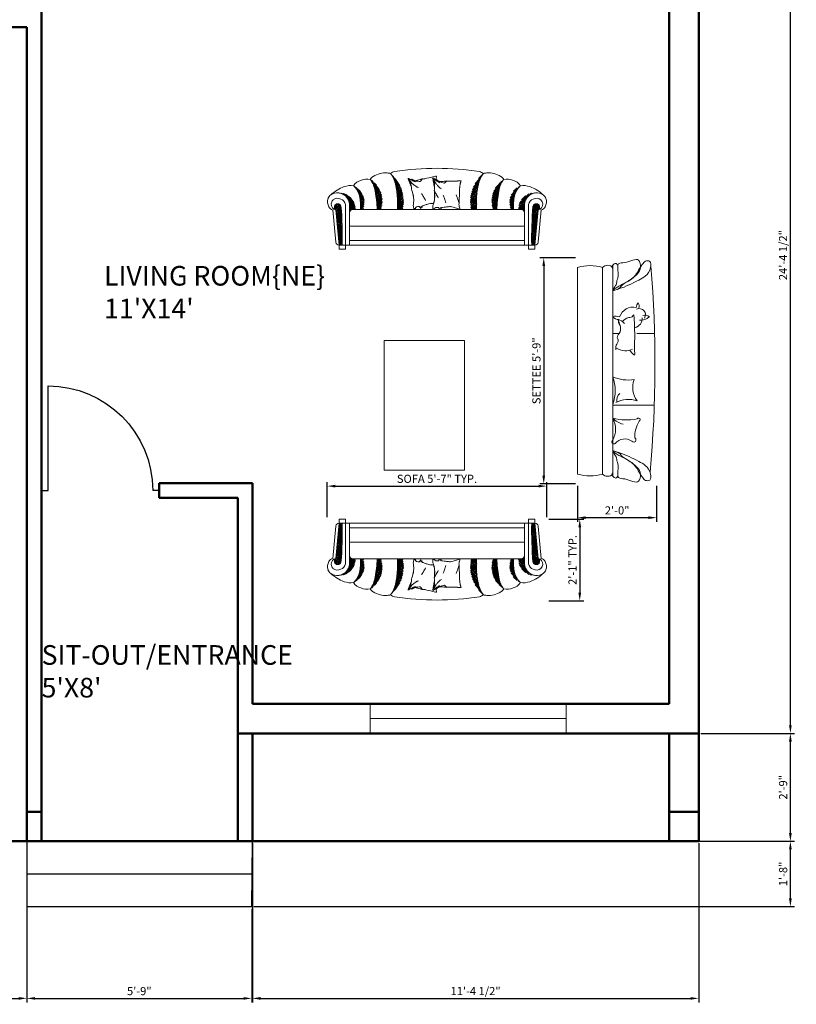
# Model space of a CAD drawing. Units: inches. Extents: x 20697 to 21575, y 6189 to 6822.
# Tile 2 of 7: x 20826 to 21063, y 6189 to 6490. Entities that reach past the tile are written whole.
import ezdxf

# ---------------------------------------------------------------- set-up
doc = ezdxf.new("R2010")
doc.units = ezdxf.units.IN
for name, color, linetype, lineweight in [('A-ANNO-DIMS', 2, 'Continuous', 18), ('A-AREA-IDEN', 7, 'Continuous', 18), ('A-DOOR', 4, 'Continuous', 25), ('A-FLOR-STRS', 3, 'Continuous', 25), ('A-FURN', 8, 'Continuous', 18), ('A-GLAZ', 4, 'Continuous', 18), ('A-WALL', 7, 'Continuous', 50)]:
    doc.layers.add(name, color=color, linetype=linetype, lineweight=lineweight)
doc.styles.get("Standard").update_dxf_attribs({"font": 'arial.ttf'})
doc.dimstyles.new('ISO-25', dxfattribs={"dimtxt": 2.5, "dimasz": 2.5, "dimexe": 1.25, "dimexo": 0.625, "dimtad": 1, "dimdec": 0, "dimlunit": 3, "dimtxsty": 'Standard', "dimcen": 2.5, "dimadec": 0, "dimazin": 0, "dimtfac": 1, "dimtdec": 0, "dimtmove": 0, "dimatfit": 3, "dimfxl": 1, "dimarcsym": 0})

# ---------------------------------------------------------------- blocks, each defined once
blk = doc.blocks.new('A$C37157CB5')
for p, q in [((460, 748), (461, 749)), ((467, 737), (471, 741)), ((489, 723), (470, 742)), ((680, 808), (681, 809)), ((687, 798), (690, 801)), ((694, 787), (699, 792)), ((710, 768), (699, 778)), ((701, 776), (708, 783)), ((706, 764), (716, 774)), ((712, 752), (724, 764)), ((719, 741), (715, 745)), ((717, 739), (732, 755)), ((721, 726), (740, 745)), ((745, 732), (723, 754)), ((1586, 707), (1643, 765)), ((1630, 731), (1615, 746)), ((1629, 750), (1620, 758)), ((1624, 763), (1670, 809)), ((1640, 757), (1633, 763)), ((1645, 769), (1636, 778)), ((1651, 780), (1651, 781)), ((1658, 791), (1654, 796)), ((1672, 812), (1672, 812)), ((1803, 660), (1885, 741)), ((1885, 741), (1882, 744)), ((284, 678), (286, 679)), ((294, 670), (286, 679)), ((292, 668), (297, 673)), ((300, 659), (308, 666)), ((308, 649), (318, 659)), ((330, 635), (308, 657)), ((315, 638), (328, 650)), ((322, 627), (337, 642)), ((474, 726), (481, 734)), ((481, 715), (491, 726)), ((498, 697), (482, 713)), ((487, 703), (500, 717)), ((492, 691), (509, 708)), ((507, 670), (496, 681)), ((497, 679), (518, 699)), ((524, 688), (502, 710)), ((502, 665), (526, 689)), ((515, 644), (505, 655)), ((506, 652), (533, 679)), ((509, 637), (540, 669)), ((533, 662), (511, 684)), ((512, 622), (547, 658)), ((514, 607), (553, 647)), ((516, 592), (559, 635)), ((542, 635), (520, 657)), ((559, 636), (546, 648)), ((728, 715), (724, 719)), ((725, 712), (747, 734)), ((728, 698), (754, 723)), ((736, 688), (729, 696)), ((731, 683), (761, 712)), ((754, 706), (732, 728)), ((745, 662), (733, 674)), ((734, 668), (767, 701)), ((737, 654), (773, 690)), ((754, 635), (738, 652)), ((740, 639), (779, 678)), ((763, 679), (741, 701)), ((742, 623), (784, 665)), ((744, 608), (789, 653)), ((746, 592), (794, 640)), ((772, 653), (750, 675)), ((781, 626), (759, 648)), ((776, 684), (767, 693)), ((789, 653), (776, 666)), ((798, 626), (785, 640)), ((1539, 572), (1610, 643)), ((1543, 593), (1614, 665)), ((1548, 617), (1619, 688)), ((1556, 642), (1624, 710)), ((1576, 626), (1557, 645)), ((1567, 653), (1562, 658)), ((1568, 671), (1631, 735)), ((1593, 644), (1571, 666)), ((1584, 670), (1573, 682)), ((1602, 617), (1580, 640)), ((1602, 688), (1585, 706)), ((1611, 662), (1589, 684)), ((1593, 715), (1591, 717)), ((1620, 706), (1598, 728)), ((1611, 644), (1598, 657)), ((1611, 732), (1605, 738)), ((1619, 689), (1607, 701)), ((1616, 674), (1615, 675)), ((1626, 718), (1624, 719)), ((1770, 573), (1843, 646)), ((1776, 596), (1850, 670)), ((1785, 624), (1861, 700)), ((1814, 617), (1792, 639)), ((1805, 644), (1798, 651)), ((1832, 635), (1810, 657)), ((1823, 662), (1812, 673)), ((1841, 679), (1827, 693)), ((1845, 657), (1828, 675)), ((1842, 643), (1836, 648)), ((1858, 697), (1844, 712)), ((1854, 683), (1845, 693)), ((1871, 719), (1862, 729)), ((1865, 708), (1863, 710)), ((1972, 580), (2046, 655)), ((1996, 622), (2034, 660)), ((2024, 620), (2008, 636)), ((2018, 644), (2016, 645)), ((2037, 642), (2026, 654)), ((2052, 662), (2046, 669)), ((2069, 681), (2068, 681)), ((122, 604), (123, 605)), ((136, 601), (140, 604)), ((153, 600), (150, 603)), ((150, 596), (156, 602)), ((162, 591), (170, 599)), ((180, 591), (172, 599)), ((174, 585), (184, 595)), ((184, 578), (196, 590)), ((215, 556), (193, 578)), ((194, 570), (208, 584)), ((206, 582), (200, 589)), ((203, 561), (219, 578)), ((211, 551), (230, 570)), ((218, 541), (240, 563)), ((241, 547), (219, 569)), ((224, 529), (222, 531)), ((223, 528), (249, 554)), ((228, 515), (257, 545)), ((250, 520), (228, 542)), ((232, 502), (265, 535)), ((277, 511), (255, 533)), ((339, 609), (323, 625)), ((327, 615), (345, 633)), ((333, 603), (353, 623)), ((348, 582), (336, 593)), ((338, 590), (360, 613)), ((342, 576), (367, 602)), ((365, 600), (343, 622)), ((356, 556), (343, 569)), ((345, 562), (373, 590)), ((347, 546), (379, 578)), ((365, 529), (347, 547)), ((349, 531), (384, 565)), ((351, 515), (388, 552)), ((374, 573), (352, 595)), ((353, 499), (391, 537)), ((383, 547), (361, 569)), ((392, 520), (370, 542)), ((524, 617), (510, 632)), ((533, 591), (513, 611)), ((519, 577), (565, 623)), ((542, 564), (520, 586)), ((521, 561), (570, 610)), ((523, 545), (574, 596)), ((524, 547), (523, 548)), ((525, 530), (578, 582)), ((527, 514), (581, 568)), ((528, 498), (583, 553)), ((551, 609), (529, 631)), ((551, 538), (529, 560)), ((530, 481), (585, 537)), ((560, 582), (538, 604)), ((560, 511), (538, 533)), ((568, 556), (546, 578)), ((571, 606), (555, 622)), ((577, 529), (555, 551)), ((578, 581), (564, 595)), ((582, 559), (573, 569)), ((585, 539), (582, 542)), ((763, 609), (741, 630)), ((748, 575), (798, 626)), ((754, 564), (748, 571)), ((749, 559), (802, 613)), ((749, 542), (806, 598)), ((749, 506), (811, 568)), ((749, 489), (813, 553)), ((763, 538), (749, 552)), ((749, 471), (815, 536)), ((772, 582), (750, 604)), ((750, 524), (809, 584)), ((772, 511), (750, 533)), ((781, 556), (759, 578)), ((789, 600), (767, 622)), ((789, 529), (767, 551)), ((798, 573), (776, 595)), ((807, 547), (785, 569)), ((805, 602), (794, 613)), ((815, 521), (794, 542)), ((809, 580), (803, 586)), ((813, 559), (812, 560)), ((1534, 514), (1603, 583)), ((1534, 497), (1601, 563)), ((1535, 532), (1605, 602)), ((1535, 480), (1600, 545)), ((1536, 551), (1607, 622)), ((1558, 538), (1537, 559)), ((1549, 564), (1539, 574)), ((1567, 582), (1545, 604)), ((1567, 511), (1545, 533)), ((1558, 609), (1549, 618)), ((1576, 556), (1554, 578)), ((1584, 600), (1562, 622)), ((1584, 529), (1562, 551)), ((1593, 573), (1571, 595)), ((1600, 548), (1580, 569)), ((1604, 598), (1589, 613)), ((1600, 531), (1589, 542)), ((1602, 582), (1598, 586)), ((1608, 629), (1607, 631)), ((1764, 532), (1835, 603)), ((1764, 514), (1832, 582)), ((1765, 497), (1829, 561)), ((1770, 538), (1765, 543)), ((1766, 552), (1838, 624)), ((1766, 481), (1826, 541)), ((1788, 556), (1770, 574)), ((1779, 582), (1773, 588)), ((1797, 529), (1774, 551)), ((1797, 600), (1782, 615)), ((1805, 573), (1783, 595)), ((1788, 626), (1787, 627)), ((1814, 547), (1792, 569)), ((1823, 591), (1801, 613)), ((1823, 520), (1801, 542)), ((1829, 567), (1810, 586)), ((1836, 613), (1819, 631)), ((1827, 551), (1819, 560)), ((1834, 598), (1828, 604)), ((1956, 512), (2005, 560)), ((1956, 494), (2001, 539)), ((1958, 531), (2010, 583)), ((1962, 553), (2020, 611)), ((1982, 538), (1963, 557)), ((1973, 564), (1968, 570)), ((1991, 511), (1969, 533)), ((1991, 582), (1978, 595)), ((2000, 556), (1978, 578)), ((2001, 537), (1987, 551)), ((2009, 600), (1992, 617)), ((2009, 581), (1995, 595)), ((2000, 626), (1999, 627)), ((2006, 567), (2004, 569)), ((2019, 607), (2013, 613)), ((2055, 469), (2148, 562)), ((2062, 494), (2162, 594)), ((2082, 532), (2124, 574)), ((2106, 520), (2087, 539)), ((2097, 547), (2095, 548)), ((2124, 538), (2104, 557)), ((2123, 520), (2110, 533)), ((2115, 564), (2114, 566)), ((2141, 556), (2124, 573)), ((2134, 545), (2128, 551)), ((2159, 573), (2146, 587)), ((2150, 564), (2146, 569)), ((2153, 567), (2187, 601)), ((2169, 581), (2163, 586)), ((2177, 591), (2171, 597)), ((2192, 593), (2185, 601)), ((2200, 597), (2208, 604)), ((2218, 602), (2216, 605)), ((2224, 603), (2226, 605)), ((75, 451), (110, 486)), ((91, 432), (75, 448)), ((82, 458), (77, 464)), ((78, 436), (124, 482)), ((85, 426), (134, 475)), ((109, 449), (87, 472)), ((91, 414), (142, 464)), ((92, 397), (144, 450)), ((100, 476), (94, 482)), ((94, 381), (145, 433)), ((118, 423), (96, 445)), ((127, 467), (108, 485)), ((135, 441), (113, 463)), ((144, 414), (122, 436)), ((144, 449), (140, 454)), ((191, 481), (191, 45)), ((233, 503), (231, 504)), ((234, 487), (272, 524)), ((241, 476), (235, 482)), ((236, 471), (279, 513)), ((236, 453), (284, 501)), ((236, 435), (289, 489)), ((236, 418), (293, 475)), ((250, 449), (236, 464)), ((236, 45), (236, 461)), ((259, 494), (237, 516)), ((257, 425), (237, 445)), ((268, 467), (246, 489)), ((277, 441), (255, 463)), ((263, 427), (296, 460)), ((286, 485), (264, 507)), ((272, 427), (264, 436)), ((270, 427), (2080, 427)), ((294, 458), (272, 480)), ((299, 437), (281, 454)), ((281, 427), (298, 444)), ((374, 503), (352, 525)), ((356, 485), (353, 488)), ((354, 482), (393, 521)), ((354, 465), (394, 505)), ((354, 448), (393, 486)), ((365, 458), (354, 469)), ((354, 430), (390, 466)), ((374, 432), (354, 451)), ((383, 476), (361, 498)), ((388, 454), (370, 472)), ((370, 427), (384, 442)), ((394, 500), (378, 516)), ((384, 440), (378, 445)), ((393, 484), (387, 489)), ((533, 520), (525, 528)), ((542, 494), (527, 509)), ((551, 467), (529, 489)), ((531, 465), (586, 520)), ((532, 448), (585, 502)), ((533, 449), (532, 451)), ((533, 432), (583, 482)), ((537, 427), (533, 432)), ((560, 441), (538, 463)), ((568, 485), (546, 507)), ((555, 427), (546, 436)), ((547, 427), (580, 461)), ((577, 458), (555, 480)), ((585, 503), (564, 525)), ((576, 442), (564, 454)), ((564, 427), (574, 437)), ((584, 487), (573, 498)), ((582, 471), (582, 472)), ((749, 454), (815, 519)), ((754, 494), (749, 499)), ((763, 467), (749, 481)), ((750, 436), (815, 502)), ((772, 441), (750, 463)), ((781, 485), (759, 507)), ((759, 427), (814, 483)), ((767, 427), (759, 436)), ((789, 458), (767, 480)), ((798, 503), (776, 525)), ((776, 427), (812, 464)), ((798, 432), (776, 454)), ((807, 476), (785, 498)), ((811, 454), (794, 472)), ((794, 427), (809, 443)), ((815, 503), (803, 516)), ((809, 439), (803, 445)), ((815, 486), (812, 489)), ((1003, 462, 12021), (1013, 456, 12021)), ((1137, 491), (1113, 493)), ((1211, 447, 12021), (1220, 439, 12021)), ((1394, 438), (1325, 458)), ((1419, 432), (1394, 438)), ((1540, 520), (1534, 526)), ((1549, 494), (1534, 509)), ((1558, 467), (1536, 489)), ((1537, 464), (1600, 527)), ((1539, 448), (1600, 510)), ((1540, 449), (1539, 451)), ((1542, 434), (1601, 492)), ((1545, 427), (1543, 429)), ((1567, 441), (1545, 463)), ((1576, 485), (1554, 507)), ((1554, 427), (1600, 474)), ((1562, 427), (1554, 436)), ((1584, 458), (1562, 480)), ((1593, 503), (1571, 525)), ((1571, 427), (1600, 456)), ((1593, 432), (1571, 454)), ((1601, 478), (1580, 498)), ((1600, 460), (1589, 472)), ((1589, 427), (1600, 438)), ((1600, 513), (1598, 516)), ((1600, 443), (1598, 445)), ((1779, 511), (1764, 526)), ((1788, 485), (1766, 507)), ((1770, 467), (1768, 469)), ((1769, 466), (1824, 521)), ((1772, 451), (1822, 501)), ((1779, 441), (1773, 447)), ((1797, 458), (1774, 480)), ((1776, 437), (1820, 482)), ((1805, 503), (1783, 525)), ((1783, 427), (1818, 462)), ((1805, 432), (1783, 454)), ((1814, 476), (1792, 498)), ((1818, 455), (1801, 472)), ((1801, 427), (1817, 443)), ((1822, 504), (1810, 516)), ((1817, 438), (1810, 445)), ((1820, 488), (1819, 489)), ((1973, 494), (1956, 511)), ((1965, 520), (1957, 527)), ((1957, 478), (1999, 519)), ((1960, 462), (1997, 500)), ((1982, 467), (1960, 489)), ((1965, 449), (1962, 452)), ((1963, 448), (1996, 481)), ((1968, 435), (1995, 462)), ((1991, 441), (1969, 463)), ((1996, 489), (1978, 507)), ((1978, 427), (1995, 445)), ((1986, 427), (1978, 436)), ((1995, 472), (1987, 480)), ((1999, 521), (1995, 525)), ((2051, 430), (2117, 495)), ((2057, 427), (2051, 434)), ((2052, 448), (2123, 520)), ((2062, 441), (2052, 451)), ((2079, 458), (2058, 480)), ((2071, 485), (2062, 494)), ((2066, 427), (2114, 475)), ((2088, 432), (2066, 454)), ((2088, 503), (2073, 518)), ((2097, 476), (2075, 498)), ((2106, 449), (2084, 472)), ((2084, 427), (2113, 457)), ((2115, 494), (2093, 516)), ((2113, 424), (2093, 445)), ((2097, 423), (2113, 439)), ((2114, 477), (2102, 489)), ((2113, 460), (2110, 463)), ((2113, 461), (2113, 45)), ((2119, 507), (2119, 507)), ((2158, 481), (2158, 45)), ((2202, 369), (2273, 440)), ((2203, 405), (2268, 471)), ((2203, 387), (2274, 458)), ((2204, 424), (2260, 479)), ((2205, 442), (2247, 485)), ((2207, 462), (2228, 484)), ((2230, 432), (2208, 454)), ((2221, 458), (2210, 469)), ((2239, 405), (2216, 427)), ((2247, 449), (2225, 472)), ((2239, 476), (2230, 484)), ((2256, 423), (2234, 445)), ((2265, 467), (2248, 485)), ((2273, 441), (2252, 463)), ((2267, 429), (2261, 436)), ((56, 422), (87, 76)), ((124, 45), (90, 422)), ((100, 405), (91, 415)), ((109, 379), (92, 395)), ((95, 365), (146, 416)), ((118, 352), (96, 374)), ((97, 349), (146, 399)), ((98, 333), (147, 382)), ((100, 335), (98, 337)), ((99, 316), (148, 365)), ((109, 308), (99, 318)), ((101, 300), (148, 347)), ((102, 284), (149, 330)), ((127, 396), (104, 419)), ((127, 326), (104, 348)), ((135, 370), (113, 392)), ((135, 299), (113, 321)), ((144, 343), (122, 366)), ((147, 394), (131, 410)), ((149, 321), (131, 339)), ((147, 376), (140, 383)), ((239, 408), (236, 411)), ((236, 400), (237, 401)), ((236, 259), (236, 394)), ((246, 418), (246, 419)), ((2106, 414), (2113, 421)), ((2113, 407), (2108, 412)), ((2112, 403), (2113, 404)), ((2113, 394), (2113, 259)), ((2199, 295), (2253, 349)), ((2199, 277), (2251, 330)), ((2200, 314), (2255, 368)), ((2201, 350), (2258, 407)), ((2201, 332), (2256, 388)), ((2212, 343), (2201, 354)), ((2221, 317), (2201, 337)), ((2203, 370), (2202, 371)), ((2221, 388), (2203, 405)), ((2212, 414), (2204, 422)), ((2230, 361), (2208, 383)), ((2239, 335), (2216, 357)), ((2247, 379), (2225, 401)), ((2247, 308), (2225, 330)), ((2226, 45), (2260, 422)), ((2254, 355), (2234, 374)), ((2258, 404), (2243, 419)), ((2252, 339), (2243, 348)), ((2256, 387), (2252, 392)), ((2262, 76), (2293, 422)), ((118, 282), (101, 298)), ((104, 268), (149, 313)), ((127, 255), (104, 277)), ((105, 251), (150, 296)), ((109, 237), (106, 240)), ((107, 235), (151, 279)), ((108, 219), (151, 262)), ((118, 211), (108, 221)), ((110, 203), (152, 245)), ((111, 187), (152, 228)), ((135, 229), (113, 251)), ((144, 273), (122, 295)), ((144, 202), (122, 224)), ((152, 248), (131, 268)), ((150, 302), (140, 312)), ((152, 229), (140, 242)), ((150, 284), (149, 286)), ((153, 211), (149, 215)), ((2102, 247), (247, 247)), ((2195, 168), (2241, 213)), ((2196, 204), (2244, 252)), ((2196, 186), (2243, 233)), ((2197, 222), (2246, 271)), ((2203, 229), (2197, 234)), ((2212, 202), (2197, 217)), ((2198, 259), (2250, 310)), ((2198, 241), (2248, 291)), ((2212, 273), (2199, 286)), ((2221, 246), (2199, 268)), ((2203, 299), (2200, 303)), ((2230, 290), (2208, 312)), ((2230, 220), (2208, 242)), ((2239, 264), (2216, 286)), ((2239, 193), (2216, 215)), ((2243, 241), (2225, 259)), ((2248, 290), (2234, 304)), ((2242, 225), (2234, 233)), ((2246, 274), (2243, 277)), ((127, 184), (110, 201)), ((113, 170), (153, 211)), ((135, 158), (113, 180)), ((114, 154), (153, 193)), ((115, 138), (154, 176)), ((118, 140), (115, 143)), ((117, 122), (154, 159)), ((127, 114), (117, 123)), ((118, 105), (155, 142)), ((120, 89), (155, 125)), ((121, 73), (156, 108)), ((144, 131), (122, 153)), ((153, 175), (131, 198)), ((153, 105), (131, 127)), ((154, 156), (140, 171)), ((155, 138), (149, 145)), ((2193, 95), (2234, 135)), ((2193, 77), (2232, 116)), ((2194, 131), (2237, 174)), ((2194, 113), (2236, 155)), ((2194, 114), (2194, 114)), ((2195, 150), (2239, 194)), ((2203, 158), (2195, 166)), ((2212, 131), (2195, 148)), ((2221, 175), (2199, 198)), ((2221, 105), (2199, 127)), ((2230, 149), (2208, 171)), ((2233, 128), (2216, 145)), ((2238, 176), (2225, 189)), ((2232, 112), (2225, 118)), ((2236, 160), (2234, 162)), ((135, 87), (118, 104)), ((144, 61), (122, 83)), ((123, 57), (156, 90)), ((124, 45), (124, 46)), ((124, 45), (191, 45)), ((124, 45), (124, 0)), ((129, 45), (157, 73)), ((142, 45), (131, 56)), ((156, 84), (140, 100)), ((146, 45), (157, 56)), ((157, 66), (149, 74)), ((191, 45), (2158, 45)), ((191, 0), (191, 45)), ((236, 95), (2113, 95)), ((2158, 45), (2226, 45)), ((2158, 45), (2158, 0)), ((2192, 59), (2230, 97)), ((2192, 45), (2192, 45)), ((2203, 87), (2193, 97)), ((2212, 61), (2193, 80)), ((2196, 45), (2229, 77)), ((2210, 45), (2199, 56)), ((2229, 79), (2208, 100)), ((2214, 45), (2227, 58)), ((2227, 63), (2216, 74)), ((2226, 47), (2225, 47)), ((2226, 0), (2226, 45)), ((124, 0), (191, 0)), ((2158, 0), (2226, 0))]:
    blk.add_line(p, q)
for centre, radius, start, end in [((1175, -2244), 3113, 81.5928, 98.4072), ((427, 569), 184, 80.3158, 111.923), ((544, 695), 103, 121.6278, 147.3132), ((231, 581), 283, 8.6182, 36.9255), ((624, 565), 255, 86.2492, 121.4484), ((629, 648), 172, 73.8948, 86.1138), ((748, 721), 117, 104.2181, 128.0845), ((456, 644), 278, 8.4037, 37.5051), ((843, 759), 21.1, 347.452, 4.9378), ((533, 583), 373, 18.5177, 27.3927), ((863, 763), 2.87, 298.8043, 347.452), ((868, 763), 1.95, 177.3472, 298.8043), ((866, 751), 10.3, 27.2619, 73.805), ((885, 709, 6010), 40.2, 77.4624, 106.5104), ((1428, 876, 6010), 569, 193.0573, 200.7575), ((868, 711), 45.7, 57.5406, 80.6815), ((883, 817), 72.1, 263.3066, 273.6689), ((-834, 135), 1815, 17.5841, 19.6497), ((2677, 961), 1802, 186.8601, 189.5557), ((892, 777), 27.5, 271.1068, 300.6613), ((856, 674, 6010), 83.3, 45.3267, 63.0636), ((1218, 1248), 585, 237.7372, 240.1004), ((768, 406), 370, 61.7627, 64.7337), ((3434, -10441), 11451, 102.2953, 102.5916), ((1084, 493), 270, 102.7452, 109.2387), ((1191, 598), 233, 138.7413, 146.5685), ((1044, 613), 145, 97.8089, 106.7223), ((1004, 752), 1.11, 182.1199, 262.5425), ((1076, 742), 73.5, 173.0191, 178.2912), ((1260, -369), 1147, 100.8734, 102.2953), ((3570, -10412), 11451, 102.2953, 102.7452), ((1109, 769), 21.1, 336.7761, 354.2618), ((771, 653), 373, 7.8417, 16.7168), ((1129, 769), 2.87, 288.1283, 336.7761), ((1220, 522), 270, 102.7452, 109.2387), ((1134, 768), 1.95, 166.6713, 288.1283), ((1130, 757), 10.3, 16.5859, 63.1291), ((1141, 711, 6010), 40.2, 66.7865, 95.8344), ((1705, 775, 6010), 569, 182.3814, 190.0816), ((1159, 818), 72.1, 252.6306, 262.993), ((-655, 467), 1815, 6.9082, 8.9737), ((1124, 717), 45.7, 46.8646, 70.0056), ((2949, 627), 1802, 176.1842, 178.8798), ((1160, 777), 27.5, 260.4309, 289.9853), ((1106, 682, 6010), 83.3, 34.6507, 52.3877), ((1163, 801), 16.2, 262.5425, 289.2387), ((1128, 764), 38, 341.9562, 356.3713), ((-597, 644), 1765, 3.4448, 3.5038), ((1230, 753), 64.4, 161.9562, 173.0191), ((1169, 786), 1.11, 182.1199, 262.5425), ((1242, 776), 73.5, 173.0191, 182.1199), ((1568, 1179), 585, 227.0612, 229.4245), ((1893, 644), 278, 142.4949, 171.5963), ((1592, 710), 130, 51.9004, 73.0092), ((1721, 648), 172, 93.8862, 106.1052), ((1726, 565), 255, 58.5516, 93.7508), ((2118, 581), 283, 143.0745, 171.3818), ((1805, 695), 103, 32.6868, 58.3722), ((1923, 569), 184, 68.077, 99.6842), ((336, 260), 442, 111.1511, 132.9844), ((249, 457), 227, 82.3776, 108.5429), ((390, 612), 132, 104.2498, 147.7714), ((121, 518), 228, 13.7801, 46.309), ((20, 520), 730, 0.506, 13.0759), ((838, 691, 9016), 62.3, 30.2153, 41.5503), ((930, 713), 45.3, 194.4995, 219.8915), ((689, 496, 9016), 305, 42.9987, 48.1274), ((662, 612), 243, 4.4384, 11.7789), ((714, 441, 9016), 329, 47.6289, 53.0518), ((892, 605, 6010), 130, 65.8228, 80.0232), ((842, 520, 9016), 189, 53.0518, 60.2054), ((900, 81), 653, 81.4776, 86.1512), ((942, 632, 9016), 41.4, 60.2054, 70.9235), ((922, 504, 9016), 168, 70.9235, 76.2375), ((1186, 707), 45.3, 183.8235, 209.2156), ((1092, 703, 9016), 62.3, 19.5393, 30.8743), ((904, 657), 243, 353.7625, 1.1029), ((909, 539, 9016), 305, 32.3228, 37.4515), ((923, 480, 9016), 329, 36.9529, 42.3759), ((1128, 608, 6010), 130, 55.1469, 69.3473), ((1063, 534, 9016), 189, 42.3759, 49.5294), ((970, 436), 370, 51.0868, 54.0577), ((1580, -10717), 11451, 91.6193, 91.9156), ((1039, 92), 653, 70.8017, 75.4752), ((1182, 625, 9016), 41.4, 49.5294, 60.2476), ((1140, 504, 9016), 168, 60.2476, 65.5616), ((1421, 546), 233, 128.0654, 135.8925), ((1296, 463), 270, 92.0692, 98.5627), ((1335, 708), 73.5, 162.3432, 167.6153), ((1279, 588), 145, 87.133, 96.0464), ((1265, 732), 1.11, 171.444, 251.8666), ((1310, -417), 1147, 90.1974, 91.6193), ((1719, -10714), 11451, 91.6193, 92.0692), ((1436, 466), 270, 92.0692, 98.5627), ((-1363, 756), 2783, 356.9074, 358.124), ((-328, 922), 1765, 351.6214, 352.8279), ((-1963, 767), 3383, 358.253, 358.2624), ((1419, 665), 0.784, 130.0781, 231.7714), ((1390, 720), 38, 331.2802, 345.6953), ((1431, 751), 16.2, 251.8666, 278.5627), ((1488, 691), 64.4, 151.2802, 162.3432), ((1504, 711), 73.5, 162.3432, 171.444), ((1435, 735), 1.11, 171.444, 251.8666), ((2329, 520), 730, 166.9241, 179.494), ((1959, 612), 132, 32.2286, 75.7502), ((2228, 518), 228, 133.691, 166.2199), ((2101, 457), 227, 71.4571, 97.6224), ((2011, 255), 448, 46.861, 68.7756), ((122, 512), 122, 163.954, 207.2009), ((84, 513), 86.4, 125.091, 157.6914), ((99, 501), 105, 80.1608, 128.0438), ((97, 486), 58.3, 131.6128, 178.5313), ((108, 471), 76.6, 63.4052, 130.83), ((100, 466), 140, 35.0024, 83.1234), ((112, 465), 80.4, 11.0436, 67.8011), ((57, 461), 179, 0, 28.1915), ((-270, 452), 624, 357.7881, 11.1171), ((-1130, 340), 1665, 3.0268, 9.7974), ((906, 629), 1.79, 65.3104, 130.8497), ((6226, 1797), 5446, 192.3608, 193.1355), ((1493, 606), 573, 181.6934, 189.2403), ((828, 566), 95, 355.484, 14.0356), ((1529, 935, 9016), 620, 212.7247, 214.5514), ((1550, 902, 9016), 620, 210.898, 212.7247), ((1573, 864, 9016), 620, 208.6683, 210.898), ((1596, 821, 9016), 620, 206.4385, 208.6683), ((1665, 964, 9016), 620, 212.7247, 214.5514), ((1146, 629), 1.79, 54.6344, 120.1738), ((1719, 498), 573, 171.0175, 178.5644), ((6591, 791), 5446, 181.6849, 182.4595), ((1058, 582), 95, 344.808, 3.3596), ((1686, 930, 9016), 620, 210.898, 212.7247), ((1709, 892, 9016), 620, 208.6683, 210.898), ((1732, 850, 9016), 620, 206.4385, 208.6683), ((1815, 814, 9016), 620, 202.0488, 203.8754), ((1830, 778, 9016), 620, 200.2221, 202.0488), ((1845, 736, 9016), 620, 197.9923, 200.2221), ((1955, 817, 9016), 620, 202.0488, 203.8754), ((1970, 781, 9016), 620, 200.2221, 202.0488), ((1985, 739, 9016), 620, 197.9923, 200.2221), ((1605, 524), 193, 167.0058, 181.3134), ((2595, 633), 1180, 181.3134, 183.1819), ((3479, 340), 1665, 170.2026, 176.9732), ((2619, 452), 624, 168.8829, 182.2119), ((2292, 461), 179, 151.8085, 180), ((2249, 466), 140, 96.8766, 144.9976), ((2237, 465), 80.4, 112.1989, 168.9564), ((2241, 471), 76.6, 49.17, 116.5948), ((2250, 501), 105, 50.3857, 99.8392), ((2252, 486), 58.3, 1.4687, 48.3872), ((2250, 501), 105, 25.2614, 50.3857), ((2228, 512), 122, 332.7991, 16.046), ((72, 486), 66.4, 207.0007, 256.1787), ((99, 482), 60.4, 174.6837, 261.4923), ((109, 453), 36.3, 16.4859, 238.4192), ((-3636, 130), 3794, 358.7163, 5.0365), ((270, 394), 33.8, 90, 180), ((1989, 486), 1240, 178.1416, 182.7056), ((666, 498), 256, 353.4963, 0.8031), ((787, 447), 135, 0.8031, 9.2403), ((966, 491), 45.4, 148.4205, 165.7819), ((851, 423), 75.9, 9.2403, 20.5127), ((932, 426), 11, 20.5127, 125.8208), ((971, 432), 28.7, 125.8208, 184.8401), ((1020, 48), 413, 95.1879, 99.2403), ((966, 427), 36.3, 16.5118, 61.8406), ((1015, 438), 13.9, 75.5311, 180.8392), ((1054, 298), 171, 99.2403, 102.854), ((1298, -222), 741, 108.9247, 111.4387), ((978, 733), 266, 287.2453, 291.4387), ((1053, 580), 98.4, 283.6331, 296.3007), ((1101, 549), 56.9, 265.1951, 281.9052), ((996, 473), 135, 350.1272, 358.5644), ((1054, 437), 75.9, 358.5644, 9.8367), ((1135, 425), 11, 9.8367, 115.1449), ((887, 545), 256, 342.8204, 350.1272), ((1180, 482), 45.4, 137.7446, 155.106), ((1174, 424), 28.7, 115.1449, 174.1641), ((1152, 37), 413, 84.5119, 88.5644), ((1168, 420), 36.3, 5.8359, 51.1647), ((1218, 421), 13.9, 64.8551, 170.1633), ((1231, 277), 171, 88.5644, 92.178), ((1374, -280), 741, 98.2487, 100.7627), ((1860, 691, 9016), 620, 195.7626, 197.9923), ((1237, 718), 266, 276.5694, 280.7627), ((1282, 554), 98.4, 272.9572, 285.6248), ((1323, 514), 56.9, 254.5192, 271.2292), ((1999, 694, 9016), 620, 195.7626, 197.9923), ((1290, 509), 123, 347.0058, 4.9984), ((1313, 454), 101, 4.9984, 15.9508), ((1440, 471), 28.4, 196.1402, 216.7652), ((1645, 464), 227, 182.6473, 188.0485), ((1419, 432), 0.77, 74.5194, 182.6473), ((360, 486), 1240, 357.2944, 1.8584), ((2080, 394), 33.8, 0, 90), ((5985, 130), 3794, 174.9635, 181.2837), ((2241, 453), 36.3, 301.5808, 163.5141), ((2251, 482), 60.4, 278.5077, 5.3163), ((2277, 486), 66.4, 283.8213, 332.9993), ((247, 259), 11.2, 180, 270), ((2102, 259), 11.3, 270, 360), ((121, 79), 34, 185.2508, 274.5466), ((2228, 79), 34, 265.4534, 354.7492)]:
    blk.add_arc(centre, radius, start, end)
blk = doc.blocks.new('A$C453F2643')
for p, q in [((714.4, 740.2), (714.4, 570.3)), ((1404, 740.9), (1404, 338)), ((714.4, 402.5), (714.4, 338)), ((2089.1, 338), (54.8, 338)), ((2068.3, 240.5), (75.6, 240.5)), ((2068.3, 0), (75.6, 0))]:
    blk.add_line(p, q)
for centre, radius, start, end in [((1016, -10516.7), 11262.3, 84.73071, 94.85459), ((593.1, 650), 57.9, 134.96265, 202.39551), ((464.1, 609), 120.3, 353.98661, 42.91759), ((447.6, 538), 55.3, 62.24213, 124.11118), ((460, 624), 59.2, 222.86904, 270.77514), ((531.2, 595.7), 58.5, 54.95495, 208.25541), ((569.5, 533.1), 88.9, 12.48799, 95.05881), ((1233.9, 749.3), 218.6, 249.6248, 306.12597), ((1600.5, 488), 252.4, 160.39126, 208.41489), ((1543.2, 586.9), 15.8, 17.39517, 243.75099), ((997.9, 469.7), 548.1, 346.09524, 10.82501), ((1714.1, 867), 316.4, 240.50711, 270.91967), ((599.3, 537.4), 141.2, 168.75965, 250.53695), ((746, 562.1), 200, 200.39751, 221.58042), ((517.8, 508.2), 145.3, 15.91745, 17.66738), ((783.3, 490.8), 378.3, 336.19158, 8.13908), ((1738.1, 540), 21.7, 305.50028, 150.58209), ((1850, 454.1), 120.5, 145.51804, 230.12795), ((664, 365.7), 118.2, 160.99472, 193.54719), ((522, 387.5), 56.4, 298.68603, 10.57738), ((597.8, 451), 56.9, 249.06277, 311.15762), ((698.8, 360.7), 123.4, 132.60586, 167.41741), ((1364.5, 484.2), 108.1, 226.59482, 275.06469), ((1384.2, 487.3), 208.6, 314.31365, 346.10416), ((123.7, 289.3), 68.6, 134.63794, 225.36206), ((1263.4, -12.7), 375.5, 69.08406, 110.91594), ((1635.6, 150.2), 215.5, 60.64717, 119.35284), ((1757, 349.8), 19.7, 216.74138, 36.74138), ((2020.1, 289.3), 68.6, 314.63794, 45.36206), ((492, 120.2), 433.4, 163.89481, 196.10519), ((1651.9, 120.2), 433.4, 343.89481, 16.10519)]:
    blk.add_arc(centre, radius, start, end)
for points, knots in [([(301.9, 338), (295.9, 358.1), (269.7, 445.5), (219.8, 548.5), (159.4, 663.3), (96.5, 705.7), (12, 709.6), (9.4, 648.8), (39.3, 630.4), (71.2, 603), (129.6, 576.6), (199.9, 519.7), (231.1, 433.5), (283.4, 406), (309.5, 317.2), (275.2, 366.4), (251.4, 403.9), (224.5, 465.2), (171.8, 539.7), (110.4, 623), (-36.6, 588.1), (37.3, 483.4), (29, 381.2), (112.4, 386.8), (163.1, 394.3), (204, 376.7), (231.1, 377.4), (260.9, 360.3), (279.9, 347.5), (293.9, 338)], [0, 0, 0, 0, 62.714896, 273.242396, 345.195178, 444.152313, 501.915975, 542.078186, 583.658309, 600.774907, 669.093529, 773.204004, 868.098945, 913.459081, 976.173976, 997.889947, 1048.310572, 1129.579434, 1187.391404, 1329.417581, 1399.76896, 1535.048248, 1595.323867, 1660.003225, 1729.532522, 1757.449721, 1789.981938, 1807.917468, 1858.941509, 1858.941509, 1858.941509, 1858.941509]), ([(1841.9, 338), (1847.9, 358.1), (1874.1, 445.5), (1924.1, 548.5), (1984.4, 663.3), (2047.3, 705.7), (2131.8, 709.6), (2134.4, 648.8), (2104.6, 630.4), (2072.6, 603), (2014.2, 576.6), (1944, 519.7), (1912.8, 433.5), (1860.5, 406), (1834.3, 317.2), (1868.6, 366.4), (1892.5, 403.9), (1919.3, 465.2), (1972.1, 539.7), (2033.4, 623), (2180.4, 588.1), (2106.5, 483.4), (2114.9, 381.2), (2031.5, 386.8), (1980.7, 394.3), (1939.8, 376.7), (1912.7, 377.4), (1882.9, 360.3), (1864, 347.5), (1850, 338)], [0, 0, 0, 0, 62.714896, 273.242396, 345.195178, 444.152313, 501.915975, 542.078186, 583.658309, 600.774907, 669.093529, 773.204004, 868.098945, 913.459081, 976.173976, 997.889947, 1048.310572, 1129.579434, 1187.391404, 1329.417581, 1399.76896, 1535.048248, 1595.323867, 1660.003225, 1729.532522, 1757.449721, 1789.981938, 1807.917468, 1858.941509, 1858.941509, 1858.941509, 1858.941509]), ([(558.5, 492.4), (559, 508), (559.6, 527.6), (528.1, 540), (558.1, 546.1), (627.5, 545.2), (754, 555), (862.6, 543.4), (902.8, 552.3), (936.6, 552.9), (903.4, 526.4), (873.2, 502.2)], [0, 0, 0, 0, 43.890402, 55.258411, 65.230876, 106.352267, 311.378998, 409.149425, 431.450323, 437.758092, 502.974641, 502.974641, 502.974641, 502.974641]), ([(864.5, 530.2), (872.8, 504.9), (890.9, 449.2), (865.3, 396), (851.4, 367.1)], [0, 0, 0, 0, 77.244602, 169.422761, 169.422761, 169.422761, 169.422761]), ([(59.3, 387.2), (48.7, 381.9), (32.1, 373.7), (44.5, 346), (66, 325.6), (85.3, 334.4), (93.3, 338)], [0, 0, 0, 0, 28.933337, 45.831315, 80.204592, 104.811589, 104.811589, 104.811589, 104.811589]), ([(578.4, 387.5), (596.9, 395.2), (634.3, 410.6), (699.2, 420.3), (741.5, 369.5), (786.7, 402.1), (823.7, 366.9), (855.8, 366.6), (870.8, 366.4)], [0, 0, 0, 0, 60.44309, 122.528656, 183.34679, 211.996789, 262.942353, 307.544136, 307.544136, 307.544136, 307.544136]), ([(2084.6, 387.2), (2095.1, 381.9), (2111.8, 373.7), (2099.3, 346), (2077.9, 325.6), (2058.6, 334.4), (2050.5, 338)], [0, 0, 0, 0, 28.933337, 45.831315, 80.204592, 104.811589, 104.811589, 104.811589, 104.811589])]:
    blk.add_open_spline(points, degree=3, knots=knots)
blk = doc.blocks.new('DOOR-SWING-36')
for p, q in [((34, 0), (34, 32)), ((0, 0), (2, 0)), ((36, 0), (34, 0))]:
    blk.add_line(p, q)
blk.add_arc((34, 0), 32, 90, 180)
blk = doc.blocks.new('WIN-60X9')
for p, q in [((0, 9), (60, 9)), ((0, 0), (0, 9)), ((60, 9), (60, 0)), ((0, 4.5), (60, 4.5)), ((60, 0), (0, 0))]:
    blk.add_line(p, q)
blk = doc.blocks.new('*D40')
at = {"layer": 'A-ANNO-DIMS', "color": 0, "lineweight": -2, "transparency": 16777216}
for p, q in [((20919.65, 6337.71), (20919.65, 6348.42)), ((20986.83, 6337.71), (20986.83, 6348.42)), ((20922.15, 6347.17), (20984.33, 6347.17))]:
    blk.add_line(p, q, dxfattribs=at)
at = {"layer": 'A-ANNO-DIMS', "color": 0, "transparency": 16777216}
for points in [[(20922.15, 6347.58), (20922.15, 6346.75), (20919.65, 6347.17)], [(20984.33, 6347.58), (20984.33, 6346.75), (20986.83, 6347.17)]]:
    blk.add_solid(points, dxfattribs=at)
at = {"layer": 'Defpoints', "color": 0, "transparency": 16777216}
for p in [(20986.83, 6347.17), (20919.65, 6337.09), (20986.83, 6337.09)]:
    blk.add_point(p, dxfattribs=at)
at = {"layer": 'A-ANNO-DIMS', "color": 0, "transparency": 16777216, "insert": (20953.24, 6349.08), "char_height": 2.5, "attachment_point": 5}
blk.add_mtext('SOFA 5\'-7" TYP.', dxfattribs=at)
blk = doc.blocks.new('*D41')
at = {"layer": 'A-ANNO-DIMS', "color": 0, "lineweight": -2, "transparency": 16777216}
for p, q in [((20987.45, 6337.09), (20998.16, 6337.09)), ((20996.91, 6334.59), (20996.91, 6314.55)), ((20987.45, 6312.05), (20998.16, 6312.05))]:
    blk.add_line(p, q, dxfattribs=at)
at = {"layer": 'A-ANNO-DIMS', "color": 0, "transparency": 16777216}
for points in [[(20996.49, 6334.59), (20997.32, 6334.59), (20996.91, 6337.09)], [(20996.49, 6314.55), (20997.32, 6314.55), (20996.91, 6312.05)]]:
    blk.add_solid(points, dxfattribs=at)
at = {"layer": 'Defpoints', "color": 0, "transparency": 16777216}
for p in [(20986.83, 6337.09), (20986.83, 6312.05), (20996.91, 6312.05)]:
    blk.add_point(p, dxfattribs=at)
at = {"layer": 'A-ANNO-DIMS', "color": 0, "transparency": 16777216, "insert": (20995.02, 6324.57), "char_height": 2.5, "attachment_point": 5, "rotation": 90}
blk.add_mtext('2\'-1" TYP.', dxfattribs=at)
blk = doc.blocks.new('*D46')
at = {"layer": 'A-ANNO-DIMS', "color": 0, "lineweight": -2, "transparency": 16777216}
for p, q in [((20995.64, 6417), (20984.65, 6417)), ((20985.9, 6414.5), (20985.9, 6350.39)), ((20995.64, 6347.89), (20984.65, 6347.89))]:
    blk.add_line(p, q, dxfattribs=at)
at = {"layer": 'A-ANNO-DIMS', "color": 0, "transparency": 16777216}
for points in [[(20985.48, 6414.5), (20986.32, 6414.5), (20985.9, 6417)], [(20985.48, 6350.39), (20986.32, 6350.39), (20985.9, 6347.89)]]:
    blk.add_solid(points, dxfattribs=at)
at = {"layer": 'Defpoints', "color": 0, "transparency": 16777216}
for p in [(20996.27, 6417), (20985.9, 6347.89), (20996.27, 6347.89)]:
    blk.add_point(p, dxfattribs=at)
at = {"layer": 'A-ANNO-DIMS', "color": 0, "transparency": 16777216, "insert": (20983.98, 6382.44), "char_height": 2.5, "attachment_point": 5, "rotation": 90}
blk.add_mtext('SETTEE 5\'-9"', dxfattribs=at)
blk = doc.blocks.new('*D47')
at = {"layer": 'A-ANNO-DIMS', "color": 0, "lineweight": -2, "transparency": 16777216}
for p, q in [((20996.27, 6347.26), (20996.27, 6336.27)), ((21020.43, 6347.26), (21020.43, 6336.27)), ((20998.77, 6337.52), (21017.93, 6337.52))]:
    blk.add_line(p, q, dxfattribs=at)
at = {"layer": 'A-ANNO-DIMS', "color": 0, "transparency": 16777216}
for points in [[(20998.77, 6337.94), (20998.77, 6337.11), (20996.27, 6337.52)], [(21017.93, 6337.94), (21017.93, 6337.11), (21020.43, 6337.52)]]:
    blk.add_solid(points, dxfattribs=at)
at = {"layer": 'Defpoints', "color": 0, "transparency": 16777216}
for p in [(20996.27, 6347.89), (21020.43, 6347.89), (21020.43, 6337.52)]:
    blk.add_point(p, dxfattribs=at)
at = {"layer": 'A-ANNO-DIMS', "color": 0, "transparency": 16777216, "insert": (21008.35, 6339.42), "char_height": 2.5, "attachment_point": 5}
blk.add_mtext('2\'-0"', dxfattribs=at)
blk = doc.blocks.new('*D52')
at = {"layer": 'A-ANNO-DIMS', "color": 0, "lineweight": -2, "transparency": 16777216}
for p, q in [((20718.29, 6237.93), (20718.29, 6189.26)), ((20827.79, 6237.93), (20827.79, 6189.26)), ((20720.79, 6190.51), (20825.29, 6190.51))]:
    blk.add_line(p, q, dxfattribs=at)
at = {"layer": 'A-ANNO-DIMS', "color": 0, "transparency": 16777216}
for points in [[(20720.79, 6190.92), (20720.79, 6190.09), (20718.29, 6190.51)], [(20825.29, 6190.92), (20825.29, 6190.09), (20827.79, 6190.51)]]:
    blk.add_solid(points, dxfattribs=at)
at = {"layer": 'Defpoints', "color": 0, "transparency": 16777216}
for p in [(20718.29, 6238.56), (20827.79, 6238.56), (20827.79, 6190.51)]:
    blk.add_point(p, dxfattribs=at)
at = {"layer": 'A-ANNO-DIMS', "color": 0, "transparency": 16777216, "insert": (20773.04, 6192.42), "char_height": 2.5, "attachment_point": 5}
blk.add_mtext('9\'-1 1/2"', dxfattribs=at)
blk = doc.blocks.new('*D53')
at = {"layer": 'A-ANNO-DIMS', "color": 0, "lineweight": -2, "transparency": 16777216}
for p, q in [((20827.79, 6217.93), (20827.79, 6189.26)), ((20896.58, 6217.93), (20896.58, 6189.26)), ((20830.29, 6190.51), (20894.08, 6190.51))]:
    blk.add_line(p, q, dxfattribs=at)
at = {"layer": 'A-ANNO-DIMS', "color": 0, "transparency": 16777216}
for points in [[(20830.29, 6190.92), (20830.29, 6190.09), (20827.79, 6190.51)], [(20894.08, 6190.92), (20894.08, 6190.09), (20896.58, 6190.51)]]:
    blk.add_solid(points, dxfattribs=at)
at = {"layer": 'Defpoints', "color": 0, "transparency": 16777216}
for p in [(20827.79, 6218.56), (20896.58, 6218.56), (20896.58, 6190.51)]:
    blk.add_point(p, dxfattribs=at)
at = {"layer": 'A-ANNO-DIMS', "color": 0, "transparency": 16777216, "insert": (20862.18, 6192.41), "char_height": 2.5, "attachment_point": 5}
blk.add_mtext('5\'-9"', dxfattribs=at)
blk = doc.blocks.new('*D54')
at = {"layer": 'A-ANNO-DIMS', "color": 0, "lineweight": -2, "transparency": 16777216}
for p, q in [((20896.79, 6237.93), (20896.79, 6189.26)), ((21033.29, 6237.93), (21033.29, 6189.26)), ((20899.29, 6190.51), (21030.79, 6190.51))]:
    blk.add_line(p, q, dxfattribs=at)
at = {"layer": 'A-ANNO-DIMS', "color": 0, "transparency": 16777216}
for points in [[(20899.29, 6190.92), (20899.29, 6190.09), (20896.79, 6190.51)], [(21030.79, 6190.92), (21030.79, 6190.09), (21033.29, 6190.51)]]:
    blk.add_solid(points, dxfattribs=at)
at = {"layer": 'Defpoints', "color": 0, "transparency": 16777216}
for p in [(20896.79, 6238.56), (21033.29, 6238.56), (21033.29, 6190.51)]:
    blk.add_point(p, dxfattribs=at)
at = {"layer": 'A-ANNO-DIMS', "color": 0, "transparency": 16777216, "insert": (20965.04, 6192.42), "char_height": 2.5, "attachment_point": 5}
blk.add_mtext('11\'-4 1/2"', dxfattribs=at)
blk = doc.blocks.new('*D55')
at = {"layer": 'A-ANNO-DIMS', "color": 0, "lineweight": -2, "transparency": 16777216}
for p, q in [((20897.42, 6238.56), (21062.59, 6238.56)), ((21061.34, 6221.06), (21061.34, 6236.06)), ((20897.2, 6218.56), (21062.59, 6218.56))]:
    blk.add_line(p, q, dxfattribs=at)
at = {"layer": 'A-ANNO-DIMS', "color": 0, "transparency": 16777216}
for points in [[(21060.93, 6236.06), (21061.76, 6236.06), (21061.34, 6238.56)], [(21060.93, 6221.06), (21061.76, 6221.06), (21061.34, 6218.56)]]:
    blk.add_solid(points, dxfattribs=at)
at = {"layer": 'Defpoints', "color": 0, "transparency": 16777216}
for p in [(20896.79, 6238.56), (21061.34, 6238.56), (20896.58, 6218.56)]:
    blk.add_point(p, dxfattribs=at)
at = {"layer": 'A-ANNO-DIMS', "color": 0, "transparency": 16777216, "insert": (21059.44, 6228.56), "char_height": 2.5, "attachment_point": 5, "rotation": 90}
blk.add_mtext('1\'-8"', dxfattribs=at)
blk = doc.blocks.new('*D56')
at = {"layer": 'A-ANNO-DIMS', "color": 0, "lineweight": -2, "transparency": 16777216}
for p, q in [((21033.92, 6271.56), (21062.59, 6271.56)), ((21061.34, 6241.06), (21061.34, 6269.06)), ((21033.92, 6238.56), (21062.59, 6238.56))]:
    blk.add_line(p, q, dxfattribs=at)
at = {"layer": 'A-ANNO-DIMS', "color": 0, "transparency": 16777216}
for points in [[(21060.93, 6269.06), (21061.76, 6269.06), (21061.34, 6271.56)], [(21060.93, 6241.06), (21061.76, 6241.06), (21061.34, 6238.56)]]:
    blk.add_solid(points, dxfattribs=at)
at = {"layer": 'Defpoints', "color": 0, "transparency": 16777216}
for p in [(21033.29, 6271.56), (21061.34, 6271.56), (21033.29, 6238.56)]:
    blk.add_point(p, dxfattribs=at)
at = {"layer": 'A-ANNO-DIMS', "color": 0, "transparency": 16777216, "insert": (21059.44, 6255.06), "char_height": 2.5, "attachment_point": 5, "rotation": 90}
blk.add_mtext('2\'-9"', dxfattribs=at)
blk = doc.blocks.new('*D57')
at = {"layer": 'A-ANNO-DIMS', "color": 0, "lineweight": -2, "transparency": 16777216}
for p, q in [((21033.92, 6564.06), (21062.59, 6564.06)), ((21061.34, 6274.06), (21061.34, 6561.56)), ((21033.92, 6271.56), (21062.59, 6271.56))]:
    blk.add_line(p, q, dxfattribs=at)
at = {"layer": 'A-ANNO-DIMS', "color": 0, "transparency": 16777216}
for points in [[(21060.93, 6561.56), (21061.76, 6561.56), (21061.34, 6564.06)], [(21060.93, 6274.06), (21061.76, 6274.06), (21061.34, 6271.56)]]:
    blk.add_solid(points, dxfattribs=at)
at = {"layer": 'Defpoints', "color": 0, "transparency": 16777216}
for p in [(21033.29, 6564.06), (21061.34, 6564.06), (21033.29, 6271.56)]:
    blk.add_point(p, dxfattribs=at)
at = {"layer": 'A-ANNO-DIMS', "color": 0, "transparency": 16777216, "insert": (21059.42, 6417.81), "char_height": 2.5, "attachment_point": 5, "rotation": 90}
blk.add_mtext('24\'-4 1/2"', dxfattribs=at)

msp = doc.modelspace()

# ---------------------------------------------------------------- linework, layer by layer
at = {"layer": 'A-FLOR-STRS'}
for p, q in [((20827.79, 6238.56), (20827.79, 6218.56)), ((20896.58, 6218.56), (20896.79, 6238.56)), ((20827.79, 6228.56), (20896.68, 6228.56)), ((20827.79, 6218.56), (20896.58, 6218.56))]:
    msp.add_line(p, q, dxfattribs=at)
at = {"layer": 'A-FURN'}
for p, q in [((20937.09, 6391.74), (20937.09, 6352)), ((20961.67, 6391.74), (20937.09, 6391.74)), ((20961.67, 6352), (20961.67, 6391.74)), ((20937.09, 6352), (20961.67, 6352))]:
    msp.add_line(p, q, dxfattribs=at)
at = {"layer": 'A-WALL'}
for p, q in [((21033.29, 6750.06), (21033.29, 6238.56)), ((21024.29, 6688.56), (21024.29, 6280.56)), ((20832.29, 6492.06), (20832.29, 6238.56)), ((20727.29, 6487.56), (20827.79, 6487.56)), ((20827.79, 6487.56), (20827.79, 6238.56)), ((20868.29, 6348.06), (20896.79, 6348.06)), ((20868.29, 6348.06), (20868.29, 6343.56)), ((20896.79, 6348.06), (20896.79, 6280.56)), ((20868.29, 6343.56), (20892.29, 6343.56)), ((20892.29, 6343.56), (20892.29, 6238.56)), ((20896.79, 6280.56), (21024.29, 6280.56)), ((20892.29, 6271.56), (21033.29, 6271.56)), ((20896.79, 6271.56), (20896.79, 6238.56)), ((21024.29, 6271.56), (21024.29, 6238.56)), ((20827.79, 6247.56), (20832.29, 6247.56)), ((21024.29, 6247.56), (21033.29, 6247.56)), ((20718.29, 6238.56), (21033.29, 6238.56))]:
    msp.add_line(p, q, dxfattribs=at)

# ---------------------------------------------------------------- block references
at = {"layer": 'A-DOOR', "extrusion": (0, 0, -1), "zscale": -1}
msp.add_blockref('DOOR-SWING-36', (-20868.29, 6345.81), dxfattribs=at)
at = {"layer": 'A-FURN', "xscale": 0.0284842962911469, "yscale": 0.0284842962911469, "zscale": 0.0284842962911469}
msp.add_blockref('A$C37157CB5', (20919.78, 6419.6), dxfattribs=at)
at = {"layer": 'A-FURN'}
for name, p, xscale, yscale, zscale, rotation in [('A$C453F2643', (20996.27, 6416.46), 0.0317308676880955, 0.0317308676880955, 0.0317308676880955, 270), ('A$C37157CB5', (20919.78, 6337.09), -0.0284842962911469, 0.0284842962911469, 0.0284842962911469, 180)]:
    msp.add_blockref(name, p, dxfattribs=dict(at, xscale=xscale, yscale=yscale, zscale=zscale, rotation=rotation))
at = {"layer": 'A-GLAZ', "rotation": 180}
msp.add_blockref('WIN-60X9', (20992.79, 6280.56), dxfattribs=at)

# ---------------------------------------------------------------- texts
at = {"layer": 'A-AREA-IDEN', "char_height": 6, "attachment_point": 1}
for s, insert in [("LIVING ROOM\\{NE\\}\\P11'X14'", (20851.4, 6414.49)), ("SIT-OUT/ENTRANCE\\P5'X8'", (20832.29, 6298.53))]:
    msp.add_mtext(s, dxfattribs=dict(at, insert=insert))

# ---------------------------------------------------------------- dimensions: what is measured, and where the dimension line sits
at = {"layer": 'A-ANNO-DIMS'}
for base, p1, p2, picture, middle in [((21061.34, 6564.06), (21033.29, 6271.56), (21033.29, 6564.06), '*D57', (21059.42, 6417.81)), ((21061.34, 6271.56), (21033.29, 6238.56), (21033.29, 6271.56), '*D56', (21059.44, 6255.06)), ((21061.34, 6238.56), (20896.58, 6218.56), (20896.79, 6238.56), '*D55', (21059.44, 6228.56))]:
    dim = msp.add_linear_dim(base=base, p1=p1, p2=p2, angle=90, dimstyle='ISO-25', override={"dimdec": 1, "dimlfac": 1, "dimrnd": 0, "dimzin": 1, "dimdsep": 46, "dimlunit": 4, "dimfrac": 2}, dxfattribs=at)
    dim.commit()
    dim.dimension.update_dxf_attribs({"geometry": picture, "text_midpoint": middle})
for base, p1, p2, text, picture, middle in [((20985.9, 6347.89), (20996.27, 6417), (20996.27, 6347.89), 'SETTEE <>', '*D46', (20983.98, 6382.44)), ((20996.91, 6312.05), (20986.83, 6337.09), (20986.83, 6312.05), '<> TYP.', '*D41', (20995.02, 6324.57))]:
    dim = msp.add_linear_dim(base=base, p1=p1, p2=p2, angle=270, text=text, dimstyle='ISO-25', override={"dimdec": 1, "dimlfac": 1, "dimrnd": 0, "dimzin": 1, "dimdsep": 46, "dimlunit": 4, "dimfrac": 2}, dxfattribs=at)
    dim.commit()
    dim.dimension.update_dxf_attribs({"geometry": picture, "text_midpoint": middle})
dim = msp.add_linear_dim(base=(20986.83, 6347.17), p1=(20919.65, 6337.09), p2=(20986.83, 6337.09), text='SOFA <> TYP.', dimstyle='ISO-25', override={"dimdec": 1, "dimlfac": 1, "dimrnd": 0, "dimzin": 1, "dimdsep": 46, "dimlunit": 4, "dimfrac": 2}, dxfattribs=at)
dim.commit()
dim.dimension.update_dxf_attribs({"geometry": '*D40', "text_midpoint": (20953.24, 6349.08)})
for base, p1, p2, picture, middle in [((21020.43, 6337.52), (20996.27, 6347.89), (21020.43, 6347.89), '*D47', (21008.35, 6339.42)), ((20827.79, 6190.51), (20718.29, 6238.56), (20827.79, 6238.56), '*D52', (20773.04, 6192.42)), ((21033.29, 6190.51), (20896.79, 6238.56), (21033.29, 6238.56), '*D54', (20965.04, 6192.42)), ((20896.58, 6190.51), (20827.79, 6218.56), (20896.58, 6218.56), '*D53', (20862.18, 6192.41))]:
    dim = msp.add_linear_dim(base=base, p1=p1, p2=p2, dimstyle='ISO-25', override={"dimdec": 1, "dimlfac": 1, "dimrnd": 0, "dimzin": 1, "dimdsep": 46, "dimlunit": 4, "dimfrac": 2}, dxfattribs=at)
    dim.commit()
    dim.dimension.update_dxf_attribs({"geometry": picture, "text_midpoint": middle})

doc.saveas('drawing.dxf')
